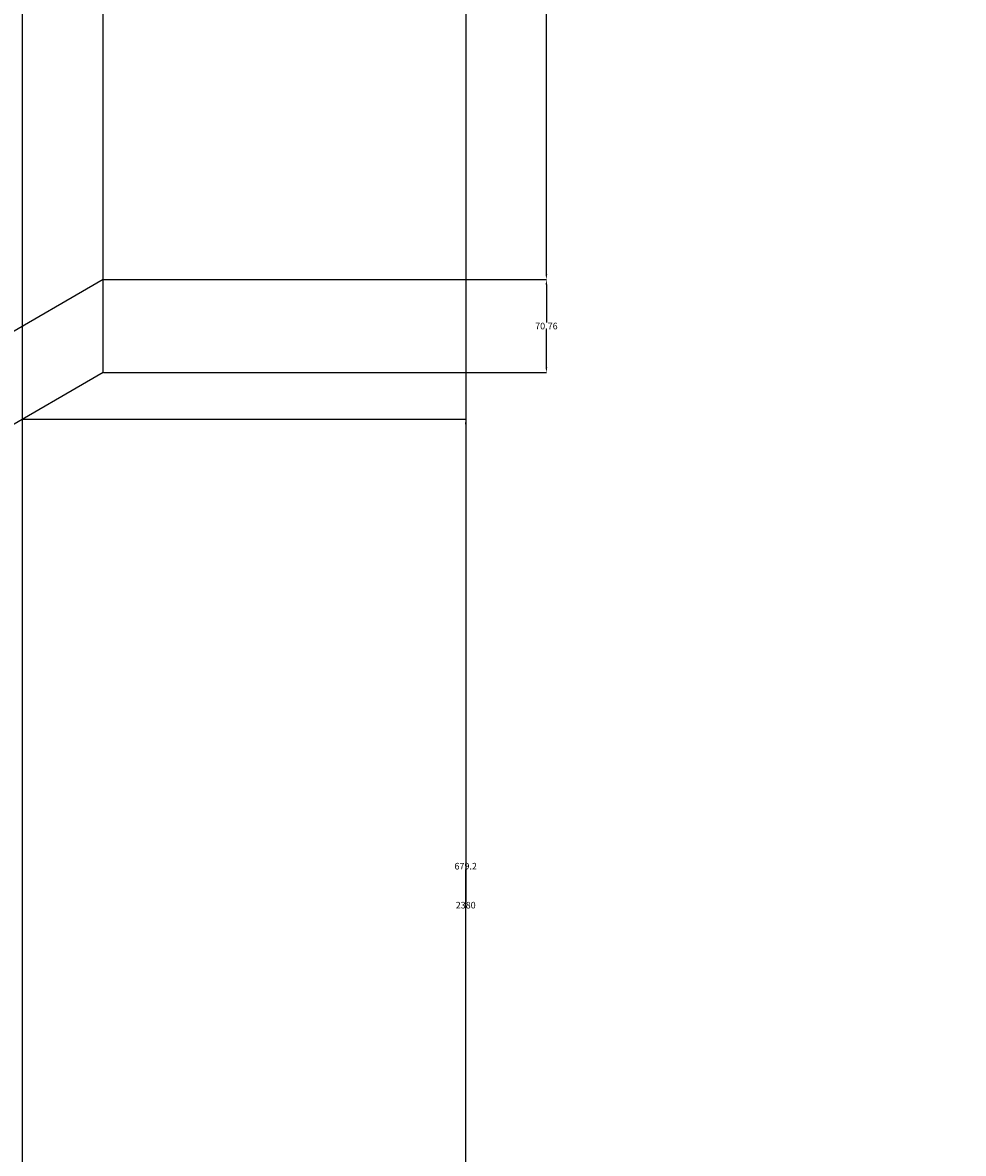
# Model space of a CAD drawing. Units: metres. Extents: x -2391 to 4922, y -635 to 4845.
# Tile 26 of 37: x 551 to 1265, y 3127 to 3986. Entities that reach past the tile are written whole.
import ezdxf

# ---------------------------------------------------------------- set-up
doc = ezdxf.new("R2010")
doc.units = ezdxf.units.M
doc.header["$MEASUREMENT"] = 0
doc.layers.add('A-ANNO-DIMS', color=2, linetype='Continuous', lineweight=18)
doc.layers.add('A-FLOR-FIXT', color=3, linetype='Continuous', lineweight=25)
doc.styles.get("Standard").update_dxf_attribs({"font": 'arial.ttf'})
doc.dimstyles.get("Standard").update_dxf_attribs({"dimtxt": 5, "dimasz": 4, "dimexe": 0.18, "dimexo": 0.0625, "dimgap": 0.09, "dimtad": 0, "dimtih": 1, "dimtoh": 1, "dimdec": 0, "dimzin": 0, "dimdsep": 46, "dimtxsty": 'Standard', "dimcen": 0.09, "dimadec": 0, "dimazin": 0, "dimtfac": 1, "dimtdec": 0, "dimtofl": 0, "dimtmove": 0, "dimatfit": 3, "dimfxl": 1, "dimtolj": 1, "dimtzin": 0, "dimarcsym": 0})

# ---------------------------------------------------------------- blocks, each defined once
blk = doc.blocks.new('*D9')
at = {"layer": 'A-ANNO-DIMS', "color": 0, "lineweight": -2, "transparency": 16777216}
for p, q in [((-2047.33, 3005.34), (-2047.33, 4841.96)), ((-2043.33, 4841.78), (-755.9, 4841.78)), ((546.74, 4841.78), (-740.69, 4841.78)), ((550.74, 4505.34), (550.74, 4841.96))]:
    blk.add_line(p, q, dxfattribs=at)
at = {"layer": 'A-ANNO-DIMS', "color": 0, "transparency": 16777216}
for points in [[(-2043.33, 4842.44), (-2043.33, 4841.11), (-2047.33, 4841.78)], [(546.74, 4842.44), (546.74, 4841.11), (550.74, 4841.78)]]:
    blk.add_solid(points, dxfattribs=at)
at = {"layer": 'Defpoints', "color": 0, "transparency": 16777216}
for p in [(550.74, 4841.78), (550.74, 4505.28), (-2047.33, 3005.28)]:
    blk.add_point(p, dxfattribs=at)
at = {"layer": 'A-ANNO-DIMS', "color": 0, "transparency": 16777216, "insert": (-748.3, 4841.78), "char_height": 5, "attachment_point": 5}
blk.add_mtext('\\A1;2598', dxfattribs=at)
blk = doc.blocks.new('*D10')
at = {"layer": 'A-ANNO-DIMS', "color": 0, "lineweight": -2, "transparency": 16777216}
for p, q in [((550.68, 4505.28), (-2384.01, 4505.28)), ((-2383.83, 4501.28), (-2383.83, 2107.92)), ((-2383.83, -290.72), (-2383.83, 2102.63)), ((-488.55, -294.72), (-2384.01, -294.72))]:
    blk.add_line(p, q, dxfattribs=at)
at = {"layer": 'A-ANNO-DIMS', "color": 0, "transparency": 16777216}
for points in [[(-2384.5, 4501.28), (-2383.17, 4501.28), (-2383.83, 4505.28)], [(-2384.5, -290.72), (-2383.17, -290.72), (-2383.83, -294.72)]]:
    blk.add_solid(points, dxfattribs=at)
at = {"layer": 'Defpoints', "color": 0, "transparency": 16777216}
for p in [(-2383.83, 4505.28), (550.74, 4505.28), (-488.49, -294.72)]:
    blk.add_point(p, dxfattribs=at)
at = {"layer": 'A-ANNO-DIMS', "color": 0, "transparency": 16777216, "insert": (-2383.83, 2105.28), "char_height": 5, "attachment_point": 5}
blk.add_mtext('\\A1;4800', dxfattribs=at)
blk = doc.blocks.new('*D11')
at = {"layer": 'A-ANNO-DIMS', "color": 0, "lineweight": -2, "transparency": 16777216}
for p, q in [((550.8, 4505.28), (887.42, 4505.28)), ((887.24, 4501.28), (887.24, 3317.92)), ((887.24, 2129.28), (887.24, 3312.63)), ((550.8, 2125.28), (887.42, 2125.28))]:
    blk.add_line(p, q, dxfattribs=at)
at = {"layer": 'A-ANNO-DIMS', "color": 0, "transparency": 16777216}
for points in [[(886.58, 4501.28), (887.91, 4501.28), (887.24, 4505.28)], [(886.58, 2129.28), (887.91, 2129.28), (887.24, 2125.28)]]:
    blk.add_solid(points, dxfattribs=at)
at = {"layer": 'Defpoints', "color": 0, "transparency": 16777216}
for p in [(550.74, 4505.28), (550.74, 2125.28), (887.24, 2125.28)]:
    blk.add_point(p, dxfattribs=at)
at = {"layer": 'A-ANNO-DIMS', "color": 0, "transparency": 16777216, "insert": (887.24, 3315.28), "char_height": 5, "attachment_point": 5}
blk.add_mtext('\\A1;2380', dxfattribs=at)
blk = doc.blocks.new('*D17')
at = {"layer": 'A-ANNO-DIMS', "color": 0, "lineweight": -2, "transparency": 16777216}
for p, q in [((550.74, 3005.34), (550.74, 4841.96)), ((554.74, 4841.78), (1014.86, 4841.78)), ((1492.03, 4841.78), (1031.91, 4841.78)), ((1496.03, 2662.52), (1496.03, 4841.96))]:
    blk.add_line(p, q, dxfattribs=at)
at = {"layer": 'A-ANNO-DIMS', "color": 0, "transparency": 16777216}
for points in [[(554.74, 4842.44), (554.74, 4841.11), (550.74, 4841.78)], [(1492.03, 4842.44), (1492.03, 4841.11), (1496.03, 4841.78)]]:
    blk.add_solid(points, dxfattribs=at)
at = {"layer": 'Defpoints', "color": 0, "transparency": 16777216}
for p in [(1496.03, 4841.78), (550.74, 3005.28), (1496.03, 2662.46)]:
    blk.add_point(p, dxfattribs=at)
at = {"layer": 'A-ANNO-DIMS', "color": 0, "transparency": 16777216, "insert": (1023.39, 4841.78), "char_height": 5, "attachment_point": 5}
blk.add_mtext('\\A1;945.3', dxfattribs=at)
blk = doc.blocks.new('*D32')
at = {"layer": 'A-ANNO-DIMS', "color": 0, "lineweight": -2, "transparency": 16777216}
for p, q in [((612.09, 4469.9), (948.7, 4469.9)), ((948.52, 4465.9), (948.52, 4132.92)), ((948.52, 3794.66), (948.52, 4127.63)), ((612.09, 3790.66), (948.7, 3790.66))]:
    blk.add_line(p, q, dxfattribs=at)
at = {"layer": 'A-ANNO-DIMS', "color": 0, "transparency": 16777216}
for points in [[(947.86, 4465.9), (949.19, 4465.9), (948.52, 4469.9)], [(947.86, 3794.66), (949.19, 3794.66), (948.52, 3790.66)]]:
    blk.add_solid(points, dxfattribs=at)
at = {"layer": 'Defpoints', "color": 0, "transparency": 16777216}
for p in [(612.02, 4469.9), (612.02, 3790.66), (948.52, 3790.66)]:
    blk.add_point(p, dxfattribs=at)
at = {"layer": 'A-ANNO-DIMS', "color": 0, "transparency": 16777216, "insert": (948.52, 4130.28), "char_height": 5, "attachment_point": 5}
blk.add_mtext('\\A1;679.2', dxfattribs=at)
blk = doc.blocks.new('*D33')
at = {"layer": 'A-ANNO-DIMS', "color": 0, "lineweight": -2, "transparency": 16777216}
for p, q in [((612.09, 3790.66), (948.7, 3790.66)), ((948.52, 3786.66), (948.52, 3757.92)), ((948.52, 3723.9), (948.52, 3752.63)), ((612.09, 3719.9), (948.7, 3719.9))]:
    blk.add_line(p, q, dxfattribs=at)
at = {"layer": 'A-ANNO-DIMS', "color": 0, "transparency": 16777216}
for points in [[(947.86, 3786.66), (949.19, 3786.66), (948.52, 3790.66)], [(947.86, 3723.9), (949.19, 3723.9), (948.52, 3719.9)]]:
    blk.add_solid(points, dxfattribs=at)
at = {"layer": 'Defpoints', "color": 0, "transparency": 16777216}
for p in [(612.02, 3790.66), (612.02, 3719.9), (948.52, 3719.9)]:
    blk.add_point(p, dxfattribs=at)
at = {"layer": 'A-ANNO-DIMS', "color": 0, "transparency": 16777216, "insert": (948.52, 3755.28), "char_height": 5, "attachment_point": 5}
blk.add_mtext('\\A1;70.76', dxfattribs=at)
blk = doc.blocks.new('*D35')
at = {"layer": 'A-ANNO-DIMS', "color": 0, "lineweight": -2, "transparency": 16777216}
for p, q in [((550.8, 3684.51), (887.42, 3684.51)), ((887.24, 3680.51), (887.24, 3347.54)), ((887.24, 3009.28), (887.24, 3342.25)), ((550.8, 3005.28), (887.42, 3005.28))]:
    blk.add_line(p, q, dxfattribs=at)
at = {"layer": 'A-ANNO-DIMS', "color": 0, "transparency": 16777216}
for points in [[(886.58, 3680.51), (887.91, 3680.51), (887.24, 3684.51)], [(886.58, 3009.28), (887.91, 3009.28), (887.24, 3005.28)]]:
    blk.add_solid(points, dxfattribs=at)
at = {"layer": 'Defpoints', "color": 0, "transparency": 16777216}
for p in [(550.74, 3684.51), (550.74, 3005.28), (887.24, 3005.28)]:
    blk.add_point(p, dxfattribs=at)
at = {"layer": 'A-ANNO-DIMS', "color": 0, "transparency": 16777216, "insert": (887.24, 3344.9), "char_height": 5, "attachment_point": 5}
blk.add_mtext('\\A1;679.2', dxfattribs=at)

msp = doc.modelspace()

# ---------------------------------------------------------------- linework, layer by layer
at = {"layer": 'A-FLOR-FIXT'}
for p, q in [((612.0233, 3719.8954), (612.0233, 4469.8954)), ((612.0233, 3790.6571), (-878.2, 2930.2763)), ((612.0233, 3719.8954), (-816.9186, 2894.8954))]:
    msp.add_line(p, q, dxfattribs=at)

# ---------------------------------------------------------------- dimensions: what is measured, and where the dimension line sits
at = {"layer": 'A-ANNO-DIMS'}
for base, p1, p2, override, picture, middle in [((550.7419, 4841.7763), (-2047.3343, 3005.2763), (550.7419, 4505.2763), {"dimdec": 0, "dimlfac": 1, "dimrnd": 0, "dimzin": 0, "dimdsep": 46, "dimlunit": 2}, '*D9', (-748.2962, 4841.7763)), ((1496.0309, 4841.7763), (550.7419, 3005.2763), (1496.0309, 2662.4566), {"dimdec": 1, "dimlfac": 1, "dimrnd": 0, "dimzin": 0, "dimdsep": 46, "dimlunit": 2}, '*D17', (1023.3864, 4841.7763))]:
    dim = msp.add_linear_dim(base=base, p1=p1, p2=p2, dimstyle='Standard', override=override, dxfattribs=at)
    dim.commit()
    dim.dimension.update_dxf_attribs({"geometry": picture, "text_midpoint": middle})
for base, p1, p2, angle, override, picture, middle in [((-2383.8343, 4505.2763), (-488.4886, -294.7237), (550.7419, 4505.2763), 90, {"dimdec": 0, "dimlfac": 1, "dimrnd": 0, "dimzin": 0, "dimdsep": 46, "dimlunit": 2}, '*D10', (-2383.8343, 2105.2763)), ((887.2419, 2125.2763), (550.7419, 4505.2763), (550.7419, 2125.2763), 270, {"dimdec": 0, "dimlfac": 1, "dimrnd": 0, "dimzin": 0, "dimdsep": 46, "dimlunit": 2}, '*D11', (887.2419, 3315.2763)), ((948.5233, 3790.6571), (612.0233, 4469.8954), (612.0233, 3790.6571), 270, {"dimdec": 1, "dimlfac": 1, "dimrnd": 0, "dimzin": 0, "dimdsep": 46, "dimlunit": 2}, '*D32', (948.5233, 4130.2763)), ((948.5233, 3719.8954), (612.0233, 3790.6571), (612.0233, 3719.8954), 270, {"dimdec": 2, "dimlfac": 1, "dimrnd": 0, "dimzin": 0, "dimdsep": 46, "dimlunit": 2}, '*D33', (948.5233, 3755.2763)), ((887.2419, 3005.2763), (550.7419, 3684.5146), (550.7419, 3005.2763), 270, {"dimdec": 1, "dimlfac": 1, "dimrnd": 0, "dimzin": 0, "dimdsep": 46, "dimlunit": 2}, '*D35', (887.2419, 3344.8954))]:
    dim = msp.add_linear_dim(base=base, p1=p1, p2=p2, angle=angle, dimstyle='Standard', override=override, dxfattribs=at)
    dim.commit()
    dim.dimension.update_dxf_attribs({"geometry": picture, "text_midpoint": middle})

doc.saveas('drawing.dxf')
